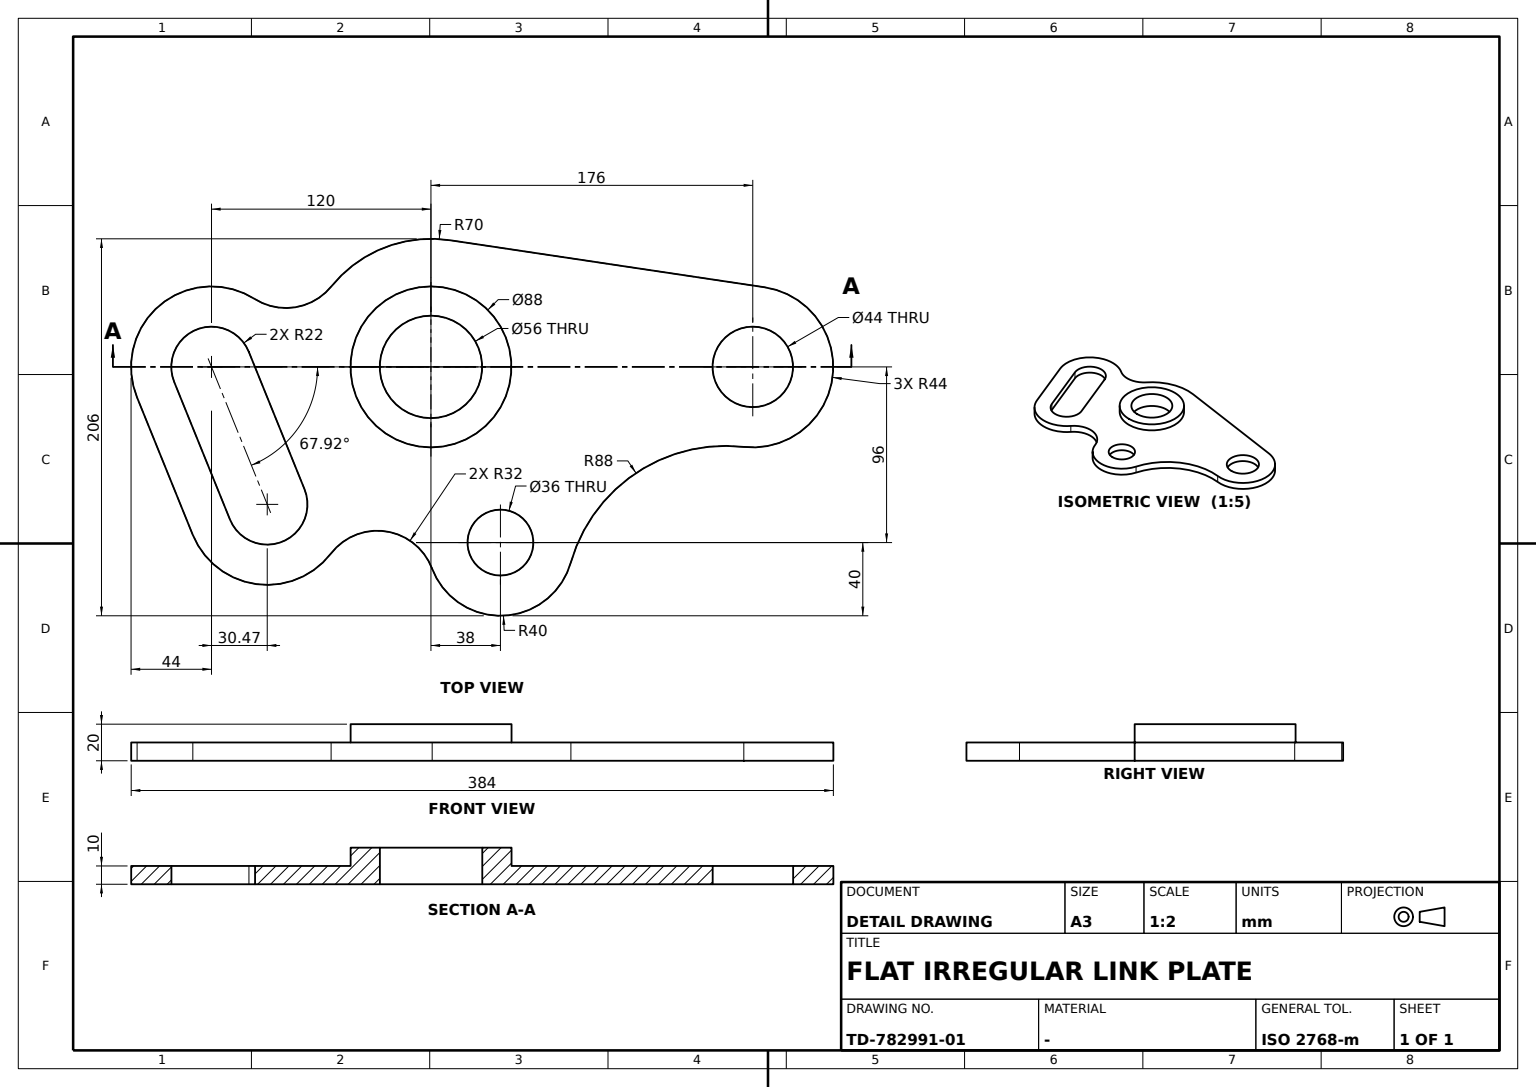
CATIA V5 part; units mm, degrees
sketch "Sketch1" plane through (0, 0, 0) normal (0, 0, 1) x (1, 0, 0)
  circle A0 centre (0, 0) radius 28
  line L0 (0, 173.7444) -> (0, -200.8937) construction
  point P0 (0, 173.7444)
  line L1 (186.7296, 0) -> (-199.2023, 0) construction
  point P1 (186.7296, 0)
  circle A1 centre (0, 176) radius 22
  point P2 (0, 176)
  arc A2 (43.718, 171.026) -> (-43.5172, 182.5) centre (0, 176) ccw
  line L2 (0, 0) -> (155.8157, -185.694) construction
  line L3 (0, -120) -> (75.1213, -89.5261) construction
  point P3 (0, -120)
  point P4 (75.1213, -89.5261)
  line L4 (-8.27, -99.6136) -> (66.8513, -69.1397)
  line L5 (83.3913, -109.9125) -> (8.27, -140.3864)
  arc A3 (66.8513, -69.1397) -> (83.3913, -109.9125) centre (75.1213, -89.5261) cw
  arc A4 (8.27, -140.3864) -> (-8.27, -99.6136) centre (0, -120) cw
  line L6 (75.1213, -89.5261) -> (0, -120) construction
  point P5 (0, -120)
  line L7 (91.6613, -130.299) -> (16.54, -160.7729)
  arc A5 (16.54, -160.7729) -> (-37.1527, -96.4272) centre (0, -120) cw
  arc A6 (101.9798, -54.6746) -> (91.6613, -130.299) centre (75.1213, -89.5261) cw
  circle A7 centre (96, 38) radius 18
  point P6 (96, 38)
  arc A8 (110.174, 0.5955) -> (106.9856, 76.4619) centre (96, 38) ccw
  arc A9 (110.174, 0.5955) -> (101.9798, -54.6746) centre (121.5132, -29.3281) ccw
  arc A10 (43.718, 171.026) -> (106.9856, 76.4619) centre (131.1539, 161.078) ccw
  line L8 (-69.232, 10.3409) -> (-43.5172, 182.5)
  arc A11 (-69.232, 10.3409) -> (-44.0402, -54.4101) centre (0, 0) ccw
  arc A12 (-44.0402, -54.4101) -> (-37.1527, -96.4272) centre (-64.1728, -79.2833) cw
  dimension "radius A0" = 28
  dimension "radius A1" = 22
  dimension "radius A2" = 44
  dimension "distance x axis P2" = 176
  dimension "angle L2 L0" = 40
  dimension "radius A4" = 22
  dimension "radius A3" = 22
  dimension "radius A6" = 44
  dimension "radius A5" = 44
  dimension "distance P5 L1" = 120
  dimension "radius A7" = 18
  dimension "radius A8" = 40
  dimension "distance P6 L1" = 38
  dimension "distance P6 L0" = 96
  dimension "length L6" = 81.0671
  dimension "angle L1 L6" = 22.081
  dimension "radius A9" = 32
  dimension "radius A10" = 88
  dimension "radius A11" = 70
  dimension "radius A12" = 32
  constraint coincidence P0 y-axis
  constraint coincidence P1 x-axis
  constraint coincidence P2 L0
  constraint coincidence P3 L0
  constraint coincidence P4 L2
  constraint vertical L0 y-axis
  constraint horizontal L1 x-axis
  constraint tangency A3 L4
  constraint tangency A4 L4
  constraint tangency A3 L5
  constraint tangency A4 L5
  constraint tangency A5 L7
  constraint tangency A6 L7
  constraint tangency A9 A8
  constraint tangency A9 A6
  constraint tangency A10 A2
  constraint tangency A10 A8
  constraint tangency L8 A2
  constraint tangency L8 A11
  constraint tangency A12 A11
  constraint tangency A12 A5
  constraint parallelism L6 L3
extrude "Pad1" add sketch "Sketch1" against normal blind 10
sketch "Sketch2" plane through (0, 0, 0) normal (0, 0, 1) x (1, 0, 0)
  circle A0 centre (0, 0) radius 44
  circle A1 centre (0, 0) radius 28
  dimension "radius A0" = 44
extrude "Pad2" add sketch "Sketch2" along normal blind 10
